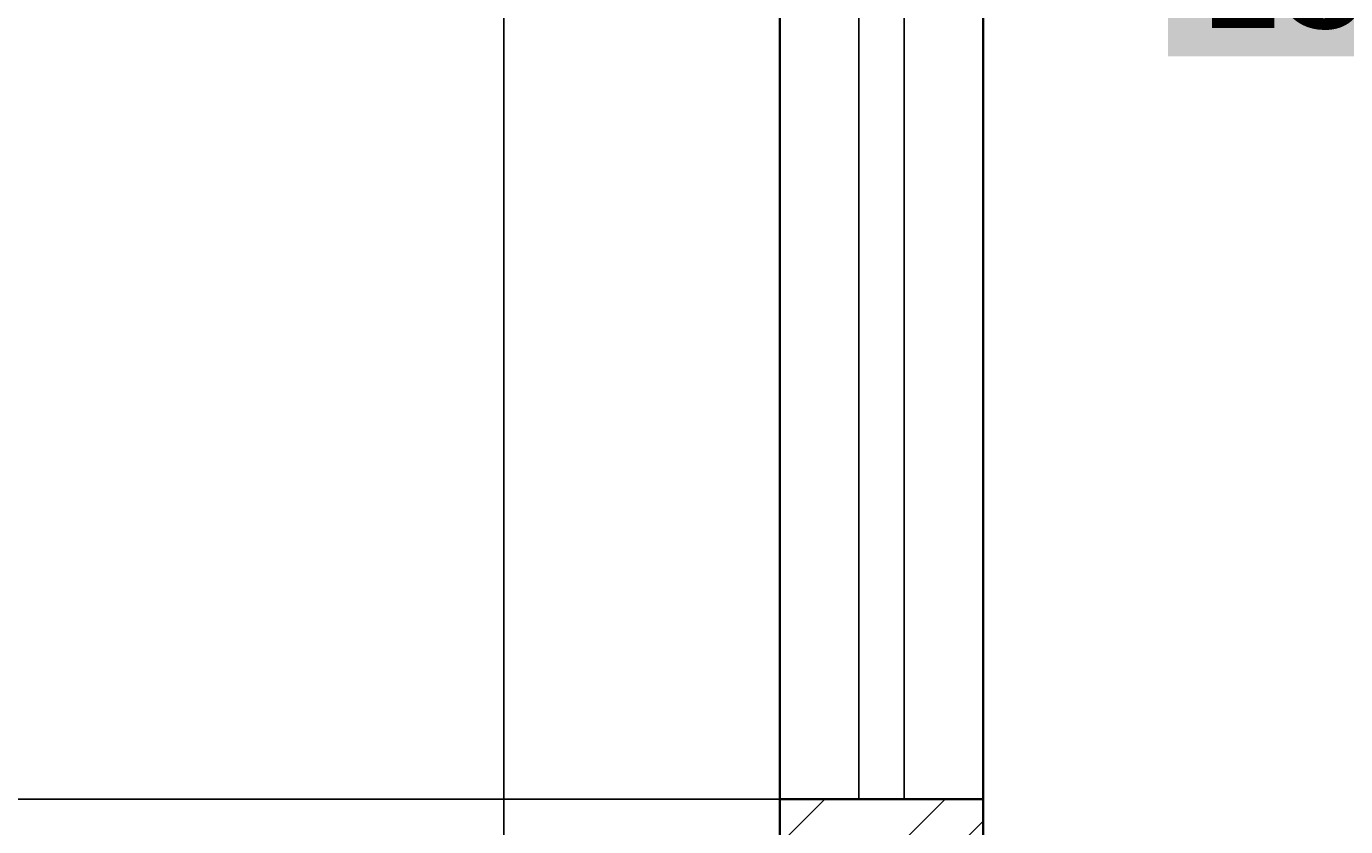
# Model space of a CAD drawing. Units: inches. Extents: x -301 to 715, y -607 to 364.
# Tile 37 of 141: x 101 to 159, y -441 to -405. Entities that reach past the tile are written whole.
import ezdxf

# ---------------------------------------------------------------- set-up
doc = ezdxf.new("R2010")
doc.units = ezdxf.units.IN
doc.header["$MEASUREMENT"] = 0
for name, color, linetype, lineweight in [('A-ANNO-DIMS', 2, 'Continuous', 18), ('A-GLAZ', 2, 'Continuous', 25), ('A-SECT', 1, 'Continuous', 35), ('A-SECT-PATT', 8, 'Continuous', 13)]:
    doc.layers.add(name, color=color, linetype=linetype, lineweight=lineweight)
doc.styles.get("Standard").update_dxf_attribs({"font": 'arial.ttf'})
doc.dimstyles.get("Standard").update_dxf_attribs({"dimtxt": 0.18, "dimasz": 0.18, "dimexe": 0.18, "dimexo": 0.0625, "dimgap": 0.09, "dimtad": 0, "dimtih": 1, "dimtoh": 1, "dimdec": 1, "dimzin": 0, "dimdsep": 46, "dimlunit": 4, "dimtxsty": 'Standard', "dimcen": 0.09, "dimclrd": 3, "dimclre": 4, "dimclrt": 6, "dimadec": 0, "dimazin": 0, "dimtfac": 1, "dimtdec": 1, "dimtofl": 0, "dimtmove": 0, "dimatfit": 3, "dimfxl": 1, "dimtfill": 2, "dimtfillclr": 51, "dimtolj": 1, "dimtzin": 0, "dimarcsym": 0})

# ---------------------------------------------------------------- blocks, each defined once
blk = doc.blocks.new('*D76')
at = {"layer": 'A-ANNO-DIMS', "color": 0, "lineweight": -2, "transparency": 16777216}
for p, q in [((158.28, -324.519), (162.311, -324.519)), ((162.131, -329.519), (162.131, -400.354)), ((162.131, -476.477), (162.131, -405.643)), ((158.28, -481.477), (162.311, -481.477))]:
    blk.add_line(p, q, dxfattribs=at)
at = {"layer": 'A-ANNO-DIMS', "color": 0, "transparency": 16777216}
for points in [[(161.297, -329.519), (162.964, -329.519), (162.131, -324.519)], [(161.297, -476.477), (162.964, -476.477), (162.131, -481.477)]]:
    blk.add_solid(points, dxfattribs=at)
at = {"layer": 'Defpoints', "color": 0, "transparency": 16777216}
for p in [(158.218, -324.519), (162.131, -324.519), (158.218, -481.477)]:
    blk.add_point(p, dxfattribs=at)
at = {"layer": 'A-ANNO-DIMS', "color": 0, "transparency": 16777216, "insert": (162.131, -402.998), "char_height": 5, "attachment_point": 5, "bg_fill": 1, "box_fill_scale": 1.25, "bg_fill_color": 51, "bg_fill_transparency": 0}
blk.add_mtext('\\A1;13\'-1"', dxfattribs=at)
blk = doc.blocks.new('*D81')
at = {"layer": 'A-ANNO-DIMS', "color": 0, "lineweight": -2, "transparency": 16777216}
for p, q in [((155.28, -385.477), (177.024, -385.477)), ((176.844, -390.477), (176.844, -430.835)), ((176.844, -476.477), (176.844, -436.12)), ((158.28, -481.477), (177.024, -481.477))]:
    blk.add_line(p, q, dxfattribs=at)
at = {"layer": 'A-ANNO-DIMS', "color": 0, "transparency": 16777216}
for points in [[(176.011, -390.477), (177.678, -390.477), (176.844, -385.477)], [(176.011, -476.477), (177.678, -476.477), (176.844, -481.477)]]:
    blk.add_solid(points, dxfattribs=at)
at = {"layer": 'Defpoints', "color": 0, "transparency": 16777216}
for p in [(155.218, -385.477), (158.218, -481.477), (176.844, -481.477)]:
    blk.add_point(p, dxfattribs=at)
at = {"layer": 'A-ANNO-DIMS', "color": 0, "transparency": 16777216, "insert": (176.844, -433.477), "char_height": 5, "attachment_point": 5, "bg_fill": 1, "box_fill_scale": 1.25, "bg_fill_color": 51, "bg_fill_transparency": 0}
blk.add_mtext("\\A1;8'", dxfattribs=at)
blk = doc.blocks.new('*D176')
at = {"layer": 'A-ANNO-DIMS', "color": 4, "lineweight": -2, "transparency": 16777216}
for p, q in [((148.28, -324.477), (215.605, -324.477)), ((-15.22, -540.477), (215.605, -540.477))]:
    blk.add_line(p, q, dxfattribs=at)
at = {"layer": 'A-ANNO-DIMS', "color": 3, "lineweight": -2, "transparency": 16777216}
for p, q in [((215.425, -324.657), (215.425, -432.296)), ((215.425, -540.297), (215.425, -432.659))]:
    blk.add_line(p, q, dxfattribs=at)
at = {"layer": 'A-ANNO-DIMS', "color": 3, "transparency": 16777216}
for points in [[(215.395, -324.657), (215.455, -324.657), (215.425, -324.477)], [(215.395, -540.297), (215.455, -540.297), (215.425, -540.477)]]:
    blk.add_solid(points, dxfattribs=at)
at = {"layer": 'Defpoints', "color": 0, "transparency": 16777216}
for p in [(148.218, -324.477), (-15.282, -540.477), (215.425, -540.477)]:
    blk.add_point(p, dxfattribs=at)
at = {"layer": 'A-ANNO-DIMS', "color": 6, "transparency": 16777216, "insert": (215.425, -432.477), "char_height": 0.18, "attachment_point": 5, "bg_fill": 1, "box_fill_scale": 1.25, "bg_fill_color": 51, "bg_fill_transparency": 0}
blk.add_mtext('\\A1;18\'-0"', dxfattribs=at)
blk = doc.blocks.new('*D187')
at = {"layer": 'A-ANNO-DIMS', "color": 4, "lineweight": -2, "transparency": 16777216}
for p, q in [((139.674, -385.477), (-266.112, -385.477)), ((143.155, -439.477), (-266.112, -439.477))]:
    blk.add_line(p, q, dxfattribs=at)
at = {"layer": 'A-ANNO-DIMS', "color": 3, "lineweight": -2, "transparency": 16777216}
for p, q in [((-265.932, -385.657), (-265.932, -412.296)), ((-265.932, -439.297), (-265.932, -412.659))]:
    blk.add_line(p, q, dxfattribs=at)
at = {"layer": 'A-ANNO-DIMS', "color": 3, "transparency": 16777216}
for points in [[(-265.962, -385.657), (-265.902, -385.657), (-265.932, -385.477)], [(-265.962, -439.297), (-265.902, -439.297), (-265.932, -439.477)]]:
    blk.add_solid(points, dxfattribs=at)
at = {"layer": 'Defpoints', "color": 0, "transparency": 16777216}
for p in [(-265.932, -385.477), (139.737, -385.477), (143.218, -439.477)]:
    blk.add_point(p, dxfattribs=at)
at = {"layer": 'A-ANNO-DIMS', "color": 6, "transparency": 16777216, "insert": (-265.932, -412.477), "char_height": 0.18, "attachment_point": 5, "bg_fill": 1, "box_fill_scale": 1.25, "bg_fill_color": 51, "bg_fill_transparency": 0}
blk.add_mtext('\\A1;4\'-6"', dxfattribs=at)
blk = doc.blocks.new('*D200')
at = {"layer": 'A-ANNO-DIMS', "color": 4, "lineweight": -2, "transparency": 16777216}
for p, q in [((412.955, -393.552), (121.926, -393.552)), ((412.955, -489.552), (121.926, -489.552))]:
    blk.add_line(p, q, dxfattribs=at)
at = {"layer": 'A-ANNO-DIMS', "color": 3, "lineweight": -2, "transparency": 16777216}
for p, q in [((122.106, -393.732), (122.106, -441.371)), ((122.106, -489.372), (122.106, -441.734))]:
    blk.add_line(p, q, dxfattribs=at)
at = {"layer": 'A-ANNO-DIMS', "color": 3, "transparency": 16777216}
for points in [[(122.076, -393.732), (122.136, -393.732), (122.106, -393.552)], [(122.076, -489.372), (122.136, -489.372), (122.106, -489.552)]]:
    blk.add_solid(points, dxfattribs=at)
at = {"layer": 'Defpoints', "color": 0, "transparency": 16777216}
for p in [(122.106, -393.552), (413.018, -393.552), (413.018, -489.552)]:
    blk.add_point(p, dxfattribs=at)
at = {"layer": 'A-ANNO-DIMS', "color": 6, "transparency": 16777216, "insert": (122.106, -441.552), "char_height": 0.18, "attachment_point": 5, "bg_fill": 1, "box_fill_scale": 1.25, "bg_fill_color": 51, "bg_fill_transparency": 0}
blk.add_mtext('\\A1;8\'-0"', dxfattribs=at)

msp = doc.modelspace()

# ---------------------------------------------------------------- hatches: boundary and pattern name
at = {"layer": 'A-SECT-PATT'}
h = msp.add_hatch(dxfattribs=at)
h.set_pattern_fill('ANSI32', color=256, scale=15)
h.set_pattern_definition([(45, (10.321, 33.8764), (-3.977476, 3.977476), []), (45, (12.973, 33.8764), (-3.977476, 3.977476), [])])
h.paths.add_polyline_path([(-35.282, -361.477), (-41.282, -361.477), (-41.282, -376.452), (-35.282, -376.452)])
h.paths.add_polyline_path([(143.218, -439.477), (134.255, -439.477), (134.255, -463.477), (143.218, -463.477)])

# ---------------------------------------------------------------- linework, layer by layer
at = {"layer": 'A-GLAZ'}
for p, q in [((137.737, -439.477), (137.737, -385.477)), ((139.737, -439.477), (139.737, -385.477))]:
    msp.add_line(p, q, dxfattribs=at)
at = {"layer": 'A-SECT'}
for p, q in [((143.218, -353.477), (143.218, -481.477)), ((134.255, -361.477), (134.255, -481.477)), ((134.255, -439.477), (143.218, -439.477))]:
    msp.add_line(p, q, dxfattribs=at)

# ---------------------------------------------------------------- dimensions: what is measured, and where the dimension line sits
at = {"layer": 'A-ANNO-DIMS'}
for base, p1, p2, override, picture, middle in [((215.425, -540.477), (148.218, -324.477), (-15.282, -540.477), {"dimdec": 1, "dimlfac": 1, "dimrnd": 0, "dimzin": 1, "dimdsep": 46, "dimlunit": 4, "dimfrac": 2}, '*D176', (215.425, -432.477)), ((162.131, -324.519), (158.218, -481.477), (158.218, -324.519), {"dimtxt": 5, "dimasz": 5, "dimclrd": 0, "dimclre": 0, "dimclrt": 0}, '*D76', (162.131, -402.998)), ((-265.932, -385.477), (143.218, -439.477), (139.737, -385.477), {"dimdec": 1, "dimlfac": 1, "dimrnd": 0, "dimzin": 1, "dimdsep": 46, "dimlunit": 4, "dimfrac": 2}, '*D187', (-265.932, -412.477)), ((176.844, -481.477), (155.218, -385.477), (158.218, -481.477), {"dimtxt": 5, "dimasz": 5, "dimclrd": 0, "dimclre": 0, "dimclrt": 0}, '*D81', (176.844, -433.477)), ((122.106, -393.552), (413.018, -489.552), (413.018, -393.552), {"dimdec": 1, "dimlfac": 1, "dimrnd": 0, "dimzin": 1, "dimdsep": 46, "dimlunit": 4, "dimfrac": 2}, '*D200', (122.106, -441.552))]:
    dim = msp.add_linear_dim(base=base, p1=p1, p2=p2, angle=90, dimstyle='Standard', override=override, dxfattribs=at)
    dim.commit()
    dim.dimension.update_dxf_attribs({"geometry": picture, "text_midpoint": middle})

doc.saveas('drawing.dxf')
